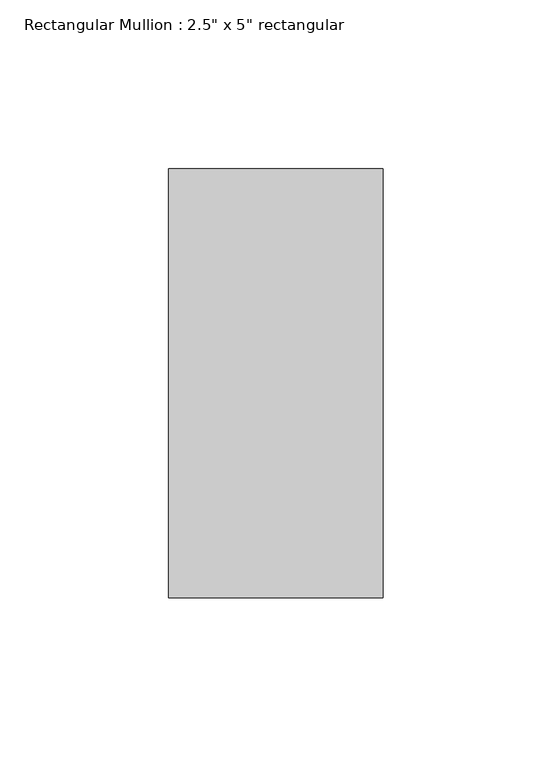
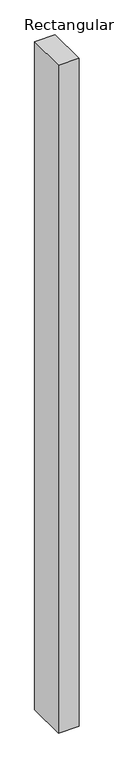
"""IFC4 building model written with IfcOpenShell, lengths in millimetres: member geometry."""

from ifc_helpers import new_model, si_unit, frame, origin, place, context, project, spatial, polyline, outline, extrude, source, transform, mapped, element, save


def member_2db96224(model_context):
    return source(origin(), model_context, "Body", "SweptSolid", [
        extrude(outline(polyline([(31.75, 63.5), (31.75, -63.5), (-31.75, -63.5), (-31.75, 63.5), (31.75, 63.5)])), frame((0.0, 0.0, -2184.4), z_axis=(0.0, 0.0, 1.0), x_axis=(1.0, 0.0, 0.0)), (0.0, 0.0, 1.0), 2184.4),
    ])


if __name__ == "__main__":
    model = new_model("IFC4")
    model_context = context("Model", 3, world=origin())
    ifc_project = project(units=[si_unit("LENGTHUNIT", "METRE", prefix="MILLI")], contexts=[model_context])
    site = spatial("IfcSite", under=ifc_project)
    building = spatial("IfcBuilding", under=site)
    placement = place(None, origin())
    member_shape = member_2db96224(model_context)
    element("IfcMember", 1, ObjectType="Rectangular Mullion : 2.5\" x 5\" rectangular", at=placement, inside=building, context=model_context, shape_type="MappedRepresentation", body=[
        mapped(member_shape, transform((0.0, 0.0, 0.0), x_axis=(1.0, 0.0, 0.0), y_axis=(0.0, 1.0, 0.0), z_axis=(0.0, 0.0, 1.0))),
    ])
    save(model, "model.ifc")

# Revit data of these elements
# Type "Rectangular Mullion : 2.5\" x 5\" rectangular"
#   built-in parameter 1007304 = 0.416667 (stored number, unit not read)
#   built-in parameter 1007301 = 0.104167 (stored number, unit not read)
#   built-in parameter 1007300 = 0.104167 (stored number, unit not read)
